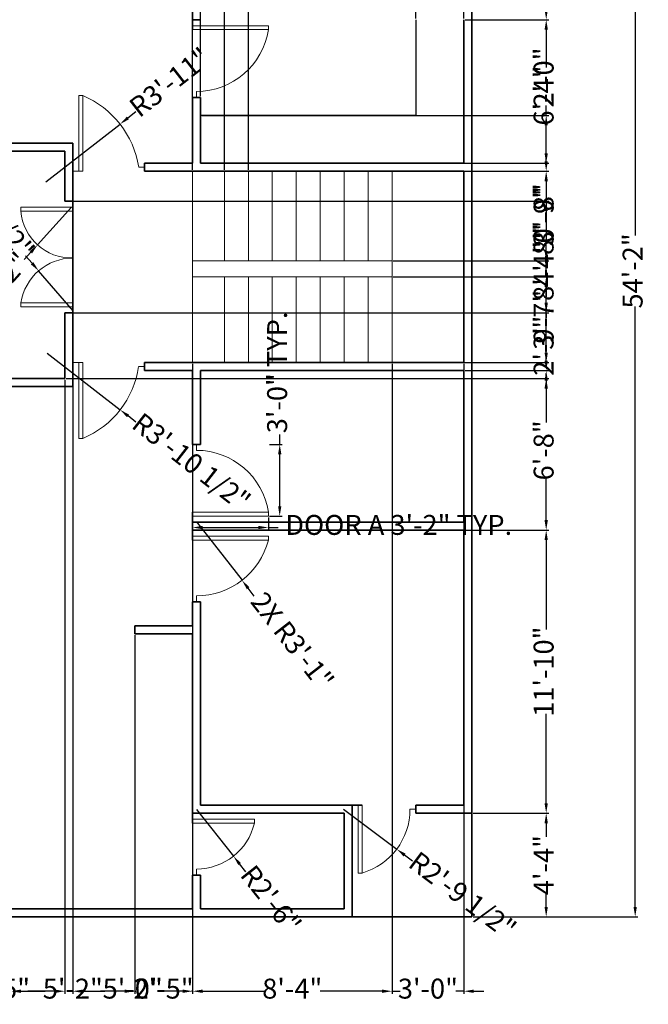
# Model space of a CAD drawing. Units: inches. Extents: x 2565 to 3182, y 2168 to 2957.
# Tile 2 of 3: x 2867 to 3182, y 2168 to 2662. Entities that reach past the tile are written whole.
import ezdxf

# ---------------------------------------------------------------- set-up
doc = ezdxf.new("R2010")
doc.units = ezdxf.units.IN
for name, color, linetype, lineweight in [('A-ANNO-DIMS', 2, 'Continuous', 13), ('A-DOOR', 4, 'Continuous', 18), ('A-FLOR-FIXT', 9, 'Continuous', 25), ('A-FLOR-STRS', 7, 'Continuous', 18), ('A-WALL', 7, 'Continuous', 35)]:
    doc.layers.add(name, color=color, linetype=linetype, lineweight=lineweight)
doc.styles.get("Standard").update_dxf_attribs({"font": 'arial.ttf'})
doc.dimstyles.new('ISO-25', dxfattribs={"dimtxt": 10, "dimasz": 5, "dimexe": 1.25, "dimexo": 0.625, "dimtad": 0, "dimdec": 0, "dimrnd": 10, "dimlunit": 3, "dimtxsty": 'Standard', "dimcen": 2.5, "dimadec": 0, "dimazin": 0, "dimtfac": 1, "dimtdec": 0, "dimtmove": 0, "dimatfit": 3, "dimfxl": 1, "dimarcsym": 0})

# ---------------------------------------------------------------- blocks, each defined once
blk = doc.blocks.new('*D2')
at = {"layer": 'A-ANNO-DIMS', "color": 0, "lineweight": -2, "transparency": 16777216}
for p, q in [((3094.05, 2859.77), (3176.57, 2859.77)), ((3175.32, 2854.77), (3175.32, 2553.57)), ((3175.32, 2216.77), (3175.32, 2517.97)), ((3094.05, 2211.77), (3176.57, 2211.77))]:
    blk.add_line(p, q, dxfattribs=at)
at = {"layer": 'A-ANNO-DIMS', "color": 0, "transparency": 16777216}
for points in [[(3174.49, 2854.77), (3176.15, 2854.77), (3175.32, 2859.77)], [(3174.49, 2216.77), (3176.15, 2216.77), (3175.32, 2211.77)]]:
    blk.add_solid(points, dxfattribs=at)
at = {"layer": 'Defpoints', "color": 0, "transparency": 16777216}
for p in [(3093.43, 2859.77), (3093.43, 2211.77), (3175.32, 2211.77)]:
    blk.add_point(p, dxfattribs=at)
at = {"layer": 'A-ANNO-DIMS', "color": 0, "transparency": 16777216, "insert": (3175.32, 2535.77), "char_height": 10, "attachment_point": 5, "rotation": 90}
blk.add_mtext('54\'-2"', dxfattribs=at)
blk = doc.blocks.new('DOOR-SWING-36-OPENING-39')
for p, q in [((2, 36), (2, 33)), ((38, 2), (0, 2)), ((0, 2), (0, 0)), ((2, 0), (38, 0)), ((38, 0), (38, 2))]:
    blk.add_line(p, q)
blk.add_arc((2, -3.4), 36.4, 8.5358, 90)
blk = doc.blocks.new('DOOR-SWING-36-OPENING-36')
for p, q in [((0, 2), (0, 38)), ((0, 38), (2, 38)), ((2, 38), (2, 0)), ((0, 0), (0, 2)), ((33, 2), (30, 2)), ((2, 0), (0, 0))]:
    blk.add_line(p, q)
blk.add_arc((-7.14, 2), 37.14, 0, 75.75)
blk = doc.blocks.new('*D7')
at = {"layer": 'A-ANNO-DIMS', "color": 0, "lineweight": -2, "transparency": 16777216}
for p, q in [((2953.43, 2412.14), (2953.43, 2405.82)), ((2991.43, 2412.14), (2991.43, 2405.82)), ((2958.43, 2407.07), (2986.43, 2407.07)), ((2991.43, 2407.07), (2996.43, 2407.07))]:
    blk.add_line(p, q, dxfattribs=at)
at = {"layer": 'A-ANNO-DIMS', "color": 0, "transparency": 16777216}
for points in [[(2958.43, 2407.9), (2958.43, 2406.23), (2953.43, 2407.07)], [(2986.43, 2407.9), (2986.43, 2406.23), (2991.43, 2407.07)]]:
    blk.add_solid(points, dxfattribs=at)
at = {"layer": 'Defpoints', "color": 0, "transparency": 16777216}
for p in [(2953.43, 2412.77), (2991.43, 2412.77), (2991.43, 2407.07)]:
    blk.add_point(p, dxfattribs=at)
at = {"layer": 'A-ANNO-DIMS', "color": 0, "transparency": 16777216, "insert": (3056.78, 2407.07), "char_height": 10, "attachment_point": 5}
blk.add_mtext('DOOR A 3\'-2" TYP.', dxfattribs=at)
blk = doc.blocks.new('*D8')
at = {"layer": 'A-ANNO-DIMS', "color": 0, "lineweight": -2, "transparency": 16777216}
for p, q in [((2997.13, 2448.77), (2997.13, 2453.77)), ((2992.05, 2448.77), (2998.38, 2448.77)), ((2997.13, 2417.77), (2997.13, 2443.77)), ((2992.05, 2412.77), (2998.38, 2412.77))]:
    blk.add_line(p, q, dxfattribs=at)
at = {"layer": 'A-ANNO-DIMS', "color": 0, "transparency": 16777216}
for points in [[(2996.3, 2443.77), (2997.96, 2443.77), (2997.13, 2448.77)], [(2996.3, 2417.77), (2997.96, 2417.77), (2997.13, 2412.77)]]:
    blk.add_solid(points, dxfattribs=at)
at = {"layer": 'Defpoints', "color": 0, "transparency": 16777216}
for p in [(2991.43, 2448.77), (2997.13, 2448.77), (2991.43, 2412.77)]:
    blk.add_point(p, dxfattribs=at)
at = {"layer": 'A-ANNO-DIMS', "color": 0, "transparency": 16777216, "insert": (2997.13, 2484.87), "char_height": 10, "attachment_point": 5, "rotation": 90}
blk.add_mtext('3\'-0" TYP.', dxfattribs=at)
blk = doc.blocks.new('*D29')
at = {"layer": 'A-ANNO-DIMS', "color": 0, "lineweight": -2, "transparency": 16777216}
for p, q in [((3094.05, 2263.77), (3131.96, 2263.77)), ((3130.71, 2258.77), (3130.71, 2251.89)), ((3130.71, 2216.77), (3130.71, 2223.65)), ((3094.05, 2211.77), (3131.96, 2211.77))]:
    blk.add_line(p, q, dxfattribs=at)
at = {"layer": 'A-ANNO-DIMS', "color": 0, "transparency": 16777216}
for points in [[(3129.88, 2258.77), (3131.54, 2258.77), (3130.71, 2263.77)], [(3129.88, 2216.77), (3131.54, 2216.77), (3130.71, 2211.77)]]:
    blk.add_solid(points, dxfattribs=at)
at = {"layer": 'Defpoints', "color": 0, "transparency": 16777216}
for p in [(3093.43, 2263.77), (3130.71, 2263.77), (3093.43, 2211.77)]:
    blk.add_point(p, dxfattribs=at)
at = {"layer": 'A-ANNO-DIMS', "color": 0, "transparency": 16777216, "insert": (3130.71, 2237.77), "char_height": 10, "attachment_point": 5, "rotation": 90}
blk.add_mtext('4\'-4"', dxfattribs=at)
blk = doc.blocks.new('*D30')
at = {"layer": 'A-ANNO-DIMS', "color": 0, "lineweight": -2, "transparency": 16777216}
for p, q in [((3090.05, 2405.77), (3131.96, 2405.77)), ((3130.71, 2400.77), (3130.71, 2355.98)), ((3130.71, 2268.77), (3130.71, 2313.55)), ((3094.05, 2263.77), (3131.96, 2263.77))]:
    blk.add_line(p, q, dxfattribs=at)
at = {"layer": 'A-ANNO-DIMS', "color": 0, "transparency": 16777216}
for points in [[(3129.88, 2400.77), (3131.54, 2400.77), (3130.71, 2405.77)], [(3129.88, 2268.77), (3131.54, 2268.77), (3130.71, 2263.77)]]:
    blk.add_solid(points, dxfattribs=at)
at = {"layer": 'Defpoints', "color": 0, "transparency": 16777216}
for p in [(3089.43, 2405.77), (3130.71, 2405.77), (3093.43, 2263.77)]:
    blk.add_point(p, dxfattribs=at)
at = {"layer": 'A-ANNO-DIMS', "color": 0, "transparency": 16777216, "insert": (3130.71, 2334.77), "char_height": 10, "attachment_point": 5, "rotation": 90}
blk.add_mtext('11\'-10"', dxfattribs=at)
blk = doc.blocks.new('*D31')
at = {"layer": 'A-ANNO-DIMS', "color": 0, "lineweight": -2, "transparency": 16777216}
for p, q in [((3090.05, 2485.77), (3131.96, 2485.77)), ((3130.71, 2480.77), (3130.71, 2459.71)), ((3130.71, 2410.77), (3130.71, 2431.82)), ((3090.05, 2405.77), (3131.96, 2405.77))]:
    blk.add_line(p, q, dxfattribs=at)
at = {"layer": 'A-ANNO-DIMS', "color": 0, "transparency": 16777216}
for points in [[(3129.88, 2480.77), (3131.54, 2480.77), (3130.71, 2485.77)], [(3129.88, 2410.77), (3131.54, 2410.77), (3130.71, 2405.77)]]:
    blk.add_solid(points, dxfattribs=at)
at = {"layer": 'Defpoints', "color": 0, "transparency": 16777216}
for p in [(3089.43, 2485.77), (3130.71, 2485.77), (3089.43, 2405.77)]:
    blk.add_point(p, dxfattribs=at)
at = {"layer": 'A-ANNO-DIMS', "color": 0, "transparency": 16777216, "insert": (3130.71, 2445.77), "char_height": 10, "attachment_point": 5, "rotation": 90}
blk.add_mtext('6\'-8"', dxfattribs=at)
blk = doc.blocks.new('*D32')
at = {"layer": 'A-ANNO-DIMS', "color": 0, "lineweight": -2, "transparency": 16777216}
for p, q in [((3090.05, 2585.77), (3131.96, 2585.77)), ((3130.71, 2580.77), (3130.71, 2549.69)), ((3130.71, 2490.77), (3130.71, 2521.84)), ((3090.05, 2485.77), (3131.96, 2485.77))]:
    blk.add_line(p, q, dxfattribs=at)
at = {"layer": 'A-ANNO-DIMS', "color": 0, "transparency": 16777216}
for points in [[(3129.88, 2580.77), (3131.54, 2580.77), (3130.71, 2585.77)], [(3129.88, 2490.77), (3131.54, 2490.77), (3130.71, 2485.77)]]:
    blk.add_solid(points, dxfattribs=at)
at = {"layer": 'Defpoints', "color": 0, "transparency": 16777216}
for p in [(3089.43, 2585.77), (3130.71, 2585.77), (3089.43, 2485.77)]:
    blk.add_point(p, dxfattribs=at)
at = {"layer": 'A-ANNO-DIMS', "color": 0, "transparency": 16777216, "insert": (3130.71, 2535.77), "char_height": 10, "attachment_point": 5, "rotation": 90}
blk.add_mtext('8\'-4"', dxfattribs=at)
blk = doc.blocks.new('*D33')
at = {"layer": 'A-ANNO-DIMS', "color": 0, "lineweight": -2, "transparency": 16777216}
for p, q in [((3090.05, 2661.77), (3131.96, 2661.77)), ((3130.71, 2656.77), (3130.71, 2637.71)), ((3130.71, 2590.77), (3130.71, 2609.82)), ((3090.05, 2585.77), (3131.96, 2585.77))]:
    blk.add_line(p, q, dxfattribs=at)
at = {"layer": 'A-ANNO-DIMS', "color": 0, "transparency": 16777216}
for points in [[(3129.88, 2656.77), (3131.54, 2656.77), (3130.71, 2661.77)], [(3129.88, 2590.77), (3131.54, 2590.77), (3130.71, 2585.77)]]:
    blk.add_solid(points, dxfattribs=at)
at = {"layer": 'Defpoints', "color": 0, "transparency": 16777216}
for p in [(3089.43, 2661.77), (3130.71, 2661.77), (3089.43, 2585.77)]:
    blk.add_point(p, dxfattribs=at)
at = {"layer": 'A-ANNO-DIMS', "color": 0, "transparency": 16777216, "insert": (3130.71, 2623.77), "char_height": 10, "attachment_point": 5, "rotation": 90}
blk.add_mtext('6\'-4"', dxfattribs=at)
blk = doc.blocks.new('*D34')
at = {"layer": 'A-ANNO-DIMS', "color": 0, "lineweight": -2, "transparency": 16777216}
for p, q in [((3090.05, 2803.77), (3131.96, 2803.77)), ((3130.71, 2798.77), (3130.71, 2753.98)), ((3130.71, 2666.77), (3130.71, 2711.55)), ((3090.05, 2661.77), (3131.96, 2661.77))]:
    blk.add_line(p, q, dxfattribs=at)
at = {"layer": 'A-ANNO-DIMS', "color": 0, "transparency": 16777216}
for points in [[(3129.88, 2798.77), (3131.54, 2798.77), (3130.71, 2803.77)], [(3129.88, 2666.77), (3131.54, 2666.77), (3130.71, 2661.77)]]:
    blk.add_solid(points, dxfattribs=at)
at = {"layer": 'Defpoints', "color": 0, "transparency": 16777216}
for p in [(3089.43, 2803.77), (3130.71, 2803.77), (3089.43, 2661.77)]:
    blk.add_point(p, dxfattribs=at)
at = {"layer": 'A-ANNO-DIMS', "color": 0, "transparency": 16777216, "insert": (3130.71, 2732.77), "char_height": 10, "attachment_point": 5, "rotation": 90}
blk.add_mtext('11\'-10"', dxfattribs=at)
blk = doc.blocks.new('*D37')
at = {"layer": 'A-ANNO-DIMS', "color": 0, "lineweight": -2, "transparency": 16777216}
for p, q in [((2924.43, 2353.14), (2924.43, 2173.24)), ((2953.43, 2353.14), (2953.43, 2173.24)), ((2919.43, 2174.49), (2914.43, 2174.49)), ((2924.43, 2174.49), (2924.93, 2174.49)), ((2953.43, 2174.49), (2952.93, 2174.49)), ((2958.43, 2174.49), (2963.43, 2174.49))]:
    blk.add_line(p, q, dxfattribs=at)
at = {"layer": 'A-ANNO-DIMS', "color": 0, "transparency": 16777216}
for points in [[(2919.43, 2175.32), (2919.43, 2173.65), (2924.43, 2174.49)], [(2958.43, 2175.32), (2958.43, 2173.65), (2953.43, 2174.49)]]:
    blk.add_solid(points, dxfattribs=at)
at = {"layer": 'Defpoints', "color": 0, "transparency": 16777216}
for p in [(2924.43, 2353.77), (2953.43, 2353.77), (2953.43, 2174.49)]:
    blk.add_point(p, dxfattribs=at)
at = {"layer": 'A-ANNO-DIMS', "color": 0, "transparency": 16777216, "insert": (2938.93, 2174.49), "char_height": 10, "attachment_point": 5}
blk.add_mtext('2\'-5"', dxfattribs=at)
blk = doc.blocks.new('*D38')
at = {"layer": 'A-ANNO-DIMS', "color": 0, "lineweight": -2, "transparency": 16777216}
for p, q in [((2862.43, 2353.14), (2862.43, 2173.24)), ((2924.43, 2353.14), (2924.43, 2173.24)), ((2867.43, 2174.49), (2879.51, 2174.49)), ((2919.43, 2174.49), (2907.35, 2174.49))]:
    blk.add_line(p, q, dxfattribs=at)
at = {"layer": 'A-ANNO-DIMS', "color": 0, "transparency": 16777216}
for points in [[(2867.43, 2175.32), (2867.43, 2173.65), (2862.43, 2174.49)], [(2919.43, 2175.32), (2919.43, 2173.65), (2924.43, 2174.49)]]:
    blk.add_solid(points, dxfattribs=at)
at = {"layer": 'Defpoints', "color": 0, "transparency": 16777216}
for p in [(2862.43, 2353.77), (2924.43, 2353.77), (2924.43, 2174.49)]:
    blk.add_point(p, dxfattribs=at)
at = {"layer": 'A-ANNO-DIMS', "color": 0, "transparency": 16777216, "insert": (2893.43, 2174.49), "char_height": 10, "attachment_point": 5}
blk.add_mtext('5\'-2"', dxfattribs=at)
blk = doc.blocks.new('*D45')
at = {"layer": 'A-ANNO-DIMS', "color": 0, "lineweight": -2, "transparency": 16777216}
for p, q in [((3130.71, 2519.77), (3130.71, 2524.77)), ((2890.05, 2514.77), (3131.96, 2514.77)), ((3130.71, 2514.77), (3130.71, 2512.27)), ((3130.71, 2481.77), (3130.71, 2484.27)), ((2890.05, 2481.77), (3131.96, 2481.77)), ((3130.71, 2476.77), (3130.71, 2471.77))]:
    blk.add_line(p, q, dxfattribs=at)
at = {"layer": 'A-ANNO-DIMS', "color": 0, "transparency": 16777216}
for points in [[(3129.88, 2519.77), (3131.54, 2519.77), (3130.71, 2514.77)], [(3129.88, 2476.77), (3131.54, 2476.77), (3130.71, 2481.77)]]:
    blk.add_solid(points, dxfattribs=at)
at = {"layer": 'Defpoints', "color": 0, "transparency": 16777216}
for p in [(2889.43, 2514.77), (3130.71, 2514.77), (2889.43, 2481.77)]:
    blk.add_point(p, dxfattribs=at)
at = {"layer": 'A-ANNO-DIMS', "color": 0, "transparency": 16777216, "insert": (3130.71, 2498.27), "char_height": 10, "attachment_point": 5, "rotation": 90}
blk.add_mtext('2\'-9"', dxfattribs=at)
blk = doc.blocks.new('*D46')
at = {"layer": 'A-ANNO-DIMS', "color": 0, "lineweight": -2, "transparency": 16777216}
for p, q in [((2890.05, 2570.77), (3131.96, 2570.77)), ((3130.71, 2565.77), (3130.71, 2556.89)), ((3130.71, 2519.77), (3130.71, 2528.65)), ((2890.05, 2514.77), (3131.96, 2514.77))]:
    blk.add_line(p, q, dxfattribs=at)
at = {"layer": 'A-ANNO-DIMS', "color": 0, "transparency": 16777216}
for points in [[(3129.88, 2565.77), (3131.54, 2565.77), (3130.71, 2570.77)], [(3129.88, 2519.77), (3131.54, 2519.77), (3130.71, 2514.77)]]:
    blk.add_solid(points, dxfattribs=at)
at = {"layer": 'Defpoints', "color": 0, "transparency": 16777216}
for p in [(2889.43, 2570.77), (3130.71, 2570.77), (2889.43, 2514.77)]:
    blk.add_point(p, dxfattribs=at)
at = {"layer": 'A-ANNO-DIMS', "color": 0, "transparency": 16777216, "insert": (3130.71, 2542.77), "char_height": 10, "attachment_point": 5, "rotation": 90}
blk.add_mtext('4\'-8"', dxfattribs=at)
blk = doc.blocks.new('*D48')
at = {"layer": 'A-ANNO-DIMS', "color": 0, "lineweight": -2, "transparency": 16777216}
for p, q in [((2824.43, 2481.14), (2824.43, 2173.24)), ((2889.43, 2481.14), (2889.43, 2173.24)), ((2829.43, 2174.49), (2843.01, 2174.49)), ((2884.43, 2174.49), (2870.85, 2174.49))]:
    blk.add_line(p, q, dxfattribs=at)
at = {"layer": 'A-ANNO-DIMS', "color": 0, "transparency": 16777216}
for points in [[(2829.43, 2175.32), (2829.43, 2173.65), (2824.43, 2174.49)], [(2884.43, 2175.32), (2884.43, 2173.65), (2889.43, 2174.49)]]:
    blk.add_solid(points, dxfattribs=at)
at = {"layer": 'Defpoints', "color": 0, "transparency": 16777216}
for p in [(2824.43, 2481.77), (2889.43, 2481.77), (2889.43, 2174.49)]:
    blk.add_point(p, dxfattribs=at)
at = {"layer": 'A-ANNO-DIMS', "color": 0, "transparency": 16777216, "insert": (2856.93, 2174.49), "char_height": 10, "attachment_point": 5}
blk.add_mtext('5\'-5"', dxfattribs=at)
blk = doc.blocks.new('*D49')
at = {"layer": 'A-ANNO-DIMS', "color": 0, "lineweight": -2, "transparency": 16777216}
for p, q in [((2893.43, 2489.14), (2893.43, 2173.24)), ((2953.43, 2489.14), (2953.43, 2173.24)), ((2898.43, 2174.49), (2909.51, 2174.49)), ((2948.43, 2174.49), (2937.35, 2174.49))]:
    blk.add_line(p, q, dxfattribs=at)
at = {"layer": 'A-ANNO-DIMS', "color": 0, "transparency": 16777216}
for points in [[(2898.43, 2175.32), (2898.43, 2173.65), (2893.43, 2174.49)], [(2948.43, 2175.32), (2948.43, 2173.65), (2953.43, 2174.49)]]:
    blk.add_solid(points, dxfattribs=at)
at = {"layer": 'Defpoints', "color": 0, "transparency": 16777216}
for p in [(2893.43, 2489.77), (2953.43, 2489.77), (2953.43, 2174.49)]:
    blk.add_point(p, dxfattribs=at)
at = {"layer": 'A-ANNO-DIMS', "color": 0, "transparency": 16777216, "insert": (2923.43, 2174.49), "char_height": 10, "attachment_point": 5}
blk.add_mtext('5\'-0"', dxfattribs=at)
blk = doc.blocks.new('*D50')
at = {"layer": 'A-ANNO-DIMS', "color": 0, "lineweight": -2, "transparency": 16777216}
for p, q in [((2953.43, 2489.14), (2953.43, 2173.24)), ((3053.43, 2489.14), (3053.43, 2173.24)), ((2958.43, 2174.49), (2989.51, 2174.49)), ((3048.43, 2174.49), (3017.35, 2174.49))]:
    blk.add_line(p, q, dxfattribs=at)
at = {"layer": 'A-ANNO-DIMS', "color": 0, "transparency": 16777216}
for points in [[(2958.43, 2175.32), (2958.43, 2173.65), (2953.43, 2174.49)], [(3048.43, 2175.32), (3048.43, 2173.65), (3053.43, 2174.49)]]:
    blk.add_solid(points, dxfattribs=at)
at = {"layer": 'Defpoints', "color": 0, "transparency": 16777216}
for p in [(2953.43, 2489.77), (3053.43, 2489.77), (3053.43, 2174.49)]:
    blk.add_point(p, dxfattribs=at)
at = {"layer": 'A-ANNO-DIMS', "color": 0, "transparency": 16777216, "insert": (3003.43, 2174.49), "char_height": 10, "attachment_point": 5}
blk.add_mtext('8\'-4"', dxfattribs=at)
blk = doc.blocks.new('*D51')
at = {"layer": 'A-ANNO-DIMS', "color": 0, "lineweight": -2, "transparency": 16777216}
for p, q in [((3053.43, 2489.14), (3053.43, 2173.24)), ((3089.43, 2489.14), (3089.43, 2173.24)), ((3048.43, 2174.49), (3043.43, 2174.49)), ((3053.43, 2174.49), (3057.52, 2174.49)), ((3089.43, 2174.49), (3085.34, 2174.49)), ((3094.43, 2174.49), (3099.43, 2174.49))]:
    blk.add_line(p, q, dxfattribs=at)
at = {"layer": 'A-ANNO-DIMS', "color": 0, "transparency": 16777216}
for points in [[(3048.43, 2175.32), (3048.43, 2173.65), (3053.43, 2174.49)], [(3094.43, 2175.32), (3094.43, 2173.65), (3089.43, 2174.49)]]:
    blk.add_solid(points, dxfattribs=at)
at = {"layer": 'Defpoints', "color": 0, "transparency": 16777216}
for p in [(3053.43, 2489.77), (3089.43, 2489.77), (3089.43, 2174.49)]:
    blk.add_point(p, dxfattribs=at)
at = {"layer": 'A-ANNO-DIMS', "color": 0, "transparency": 16777216, "insert": (3071.43, 2174.49), "char_height": 10, "attachment_point": 5}
blk.add_mtext('3\'-0"', dxfattribs=at)
blk = doc.blocks.new('*D52')
at = {"layer": 'A-ANNO-DIMS', "color": 0, "lineweight": -2, "transparency": 16777216}
for p, q in [((2953.43, 2586.39), (2953.43, 2898.3)), ((2958.43, 2897.05), (2964.43, 2897.05)), ((2969.43, 2586.39), (2969.43, 2898.3)), ((2969.43, 2897.05), (2974.43, 2897.05))]:
    blk.add_line(p, q, dxfattribs=at)
at = {"layer": 'A-ANNO-DIMS', "color": 0, "transparency": 16777216}
for points in [[(2958.43, 2897.88), (2958.43, 2896.21), (2953.43, 2897.05)], [(2964.43, 2897.88), (2964.43, 2896.21), (2969.43, 2897.05)]]:
    blk.add_solid(points, dxfattribs=at)
at = {"layer": 'Defpoints', "color": 0, "transparency": 16777216}
for p in [(2969.43, 2897.05), (2953.43, 2585.77), (2969.43, 2585.77)]:
    blk.add_point(p, dxfattribs=at)
at = {"layer": 'A-ANNO-DIMS', "color": 0, "transparency": 16777216, "insert": (2987.87, 2897.05), "char_height": 10, "attachment_point": 5}
blk.add_mtext('1\'-4"', dxfattribs=at)
blk = doc.blocks.new('*D53')
at = {"layer": 'A-ANNO-DIMS', "color": 0, "lineweight": -2, "transparency": 16777216}
for p, q in [((2969.43, 2586.39), (2969.43, 2898.3)), ((2974.43, 2897.05), (2976.43, 2897.05)), ((2981.43, 2586.39), (2981.43, 2898.3)), ((2981.43, 2897.05), (2986.43, 2897.05))]:
    blk.add_line(p, q, dxfattribs=at)
at = {"layer": 'A-ANNO-DIMS', "color": 0, "transparency": 16777216}
for points in [[(2974.43, 2897.88), (2974.43, 2896.21), (2969.43, 2897.05)], [(2976.43, 2897.88), (2976.43, 2896.21), (2981.43, 2897.05)]]:
    blk.add_solid(points, dxfattribs=at)
at = {"layer": 'Defpoints', "color": 0, "transparency": 16777216}
for p in [(2981.43, 2897.05), (2969.43, 2585.77), (2981.43, 2585.77)]:
    blk.add_point(p, dxfattribs=at)
at = {"layer": 'A-ANNO-DIMS', "color": 0, "transparency": 16777216, "insert": (2999.87, 2897.05), "char_height": 10, "attachment_point": 5}
blk.add_mtext('1\'-0"', dxfattribs=at)
blk = doc.blocks.new('*D54')
at = {"layer": 'A-ANNO-DIMS', "color": 0, "lineweight": -2, "transparency": 16777216}
for p, q in [((3054.05, 2532.77), (3131.96, 2532.77)), ((3130.71, 2527.77), (3130.71, 2525.18)), ((3130.71, 2494.77), (3130.71, 2497.36)), ((3054.05, 2489.77), (3131.96, 2489.77))]:
    blk.add_line(p, q, dxfattribs=at)
at = {"layer": 'A-ANNO-DIMS', "color": 0, "transparency": 16777216}
for points in [[(3129.88, 2527.77), (3131.54, 2527.77), (3130.71, 2532.77)], [(3129.88, 2494.77), (3131.54, 2494.77), (3130.71, 2489.77)]]:
    blk.add_solid(points, dxfattribs=at)
at = {"layer": 'Defpoints', "color": 0, "transparency": 16777216}
for p in [(3053.43, 2532.77), (3130.71, 2532.77), (3053.43, 2489.77)]:
    blk.add_point(p, dxfattribs=at)
at = {"layer": 'A-ANNO-DIMS', "color": 0, "transparency": 16777216, "insert": (3130.71, 2511.27), "char_height": 10, "attachment_point": 5, "rotation": 90}
blk.add_mtext('3\'-7"', dxfattribs=at)
blk = doc.blocks.new('*D55')
at = {"layer": 'A-ANNO-DIMS', "color": 0, "lineweight": -2, "transparency": 16777216}
for p, q in [((3130.71, 2545.77), (3130.71, 2550.77)), ((3054.05, 2540.77), (3131.96, 2540.77)), ((3130.71, 2532.77), (3130.71, 2540.77)), ((3054.05, 2532.77), (3131.96, 2532.77)), ((3130.71, 2527.77), (3130.71, 2522.77))]:
    blk.add_line(p, q, dxfattribs=at)
at = {"layer": 'A-ANNO-DIMS', "color": 0, "transparency": 16777216}
for points in [[(3129.88, 2545.77), (3131.54, 2545.77), (3130.71, 2540.77)], [(3129.88, 2527.77), (3131.54, 2527.77), (3130.71, 2532.77)]]:
    blk.add_solid(points, dxfattribs=at)
at = {"layer": 'Defpoints', "color": 0, "transparency": 16777216}
for p in [(3053.43, 2540.77), (3130.71, 2540.77), (3053.43, 2532.77)]:
    blk.add_point(p, dxfattribs=at)
at = {"layer": 'A-ANNO-DIMS', "color": 0, "transparency": 16777216, "insert": (3130.71, 2564.68), "char_height": 10, "attachment_point": 5, "rotation": 90}
blk.add_mtext('0\'-8"', dxfattribs=at)
blk = doc.blocks.new('*D56')
at = {"layer": 'A-ANNO-DIMS', "color": 0, "lineweight": -2, "transparency": 16777216}
for p, q in [((3054.05, 2585.77), (3131.96, 2585.77)), ((3130.71, 2580.77), (3130.71, 2577.18)), ((3130.71, 2545.77), (3130.71, 2549.36)), ((3054.05, 2540.77), (3131.96, 2540.77))]:
    blk.add_line(p, q, dxfattribs=at)
at = {"layer": 'A-ANNO-DIMS', "color": 0, "transparency": 16777216}
for points in [[(3129.88, 2580.77), (3131.54, 2580.77), (3130.71, 2585.77)], [(3129.88, 2545.77), (3131.54, 2545.77), (3130.71, 2540.77)]]:
    blk.add_solid(points, dxfattribs=at)
at = {"layer": 'Defpoints', "color": 0, "transparency": 16777216}
for p in [(3053.43, 2585.77), (3130.71, 2585.77), (3053.43, 2540.77)]:
    blk.add_point(p, dxfattribs=at)
at = {"layer": 'A-ANNO-DIMS', "color": 0, "transparency": 16777216, "insert": (3130.71, 2563.27), "char_height": 10, "attachment_point": 5, "rotation": 90}
blk.add_mtext('3\'-9"', dxfattribs=at)
blk = doc.blocks.new('*D57')
at = {"layer": 'A-ANNO-DIMS', "color": 0, "lineweight": -2, "transparency": 16777216}
for p, q in [((3065.43, 2662.39), (3065.43, 2898.3)), ((3070.43, 2897.05), (3084.43, 2897.05)), ((3089.43, 2662.39), (3089.43, 2898.3)), ((3089.43, 2897.05), (3094.43, 2897.05))]:
    blk.add_line(p, q, dxfattribs=at)
at = {"layer": 'A-ANNO-DIMS', "color": 0, "transparency": 16777216}
for points in [[(3070.43, 2897.88), (3070.43, 2896.21), (3065.43, 2897.05)], [(3084.43, 2897.88), (3084.43, 2896.21), (3089.43, 2897.05)]]:
    blk.add_solid(points, dxfattribs=at)
at = {"layer": 'Defpoints', "color": 0, "transparency": 16777216}
for p in [(3089.43, 2897.05), (3065.43, 2661.77), (3089.43, 2661.77)]:
    blk.add_point(p, dxfattribs=at)
at = {"layer": 'A-ANNO-DIMS', "color": 0, "transparency": 16777216, "insert": (3108.43, 2897.05), "char_height": 10, "attachment_point": 5}
blk.add_mtext('2\'-0"', dxfattribs=at)
blk = doc.blocks.new('*D58')
at = {"layer": 'A-ANNO-DIMS', "color": 0, "lineweight": -2, "transparency": 16777216}
for p, q in [((3130.71, 2613.77), (3130.71, 2618.77)), ((2958.05, 2613.77), (3131.96, 2613.77)), ((3130.71, 2594.77), (3130.71, 2608.77)), ((2958.05, 2589.77), (3131.96, 2589.77))]:
    blk.add_line(p, q, dxfattribs=at)
at = {"layer": 'A-ANNO-DIMS', "color": 0, "transparency": 16777216}
for points in [[(3129.88, 2608.77), (3131.54, 2608.77), (3130.71, 2613.77)], [(3129.88, 2594.77), (3131.54, 2594.77), (3130.71, 2589.77)]]:
    blk.add_solid(points, dxfattribs=at)
at = {"layer": 'Defpoints', "color": 0, "transparency": 16777216}
for p in [(2957.43, 2613.77), (3130.71, 2613.77), (2957.43, 2589.77)]:
    blk.add_point(p, dxfattribs=at)
at = {"layer": 'A-ANNO-DIMS', "color": 0, "transparency": 16777216, "insert": (3130.71, 2632.77), "char_height": 10, "attachment_point": 5, "rotation": 90}
blk.add_mtext('2\'-0"', dxfattribs=at)
blk = doc.blocks.new('*D59')
at = {"layer": 'A-ANNO-DIMS', "color": 0, "lineweight": -2, "transparency": 16777216}
for p, q in [((2948.43, 2897.05), (2943.43, 2897.05)), ((2953.43, 2623.39), (2953.43, 2898.3)), ((2953.43, 2897.05), (2957.43, 2897.05)), ((2957.43, 2623.39), (2957.43, 2898.3)), ((2962.43, 2897.05), (2967.43, 2897.05))]:
    blk.add_line(p, q, dxfattribs=at)
at = {"layer": 'A-ANNO-DIMS', "color": 0, "transparency": 16777216}
for points in [[(2948.43, 2897.88), (2948.43, 2896.21), (2953.43, 2897.05)], [(2962.43, 2897.88), (2962.43, 2896.21), (2957.43, 2897.05)]]:
    blk.add_solid(points, dxfattribs=at)
at = {"layer": 'Defpoints', "color": 0, "transparency": 16777216}
for p in [(2957.43, 2897.05), (2953.43, 2622.77), (2957.43, 2622.77)]:
    blk.add_point(p, dxfattribs=at)
at = {"layer": 'A-ANNO-DIMS', "color": 0, "transparency": 16777216, "insert": (2981.35, 2897.05), "char_height": 10, "attachment_point": 5}
blk.add_mtext('0\'-4"', dxfattribs=at)
blk = doc.blocks.new('*D60')
at = {"layer": 'A-ANNO-DIMS', "color": 0, "lineweight": -2, "transparency": 16777216}
for p, q in [((2924.97, 2615.52), (2921.02, 2612.45)), ((2879.89, 2580.46), (2917.08, 2609.38))]:
    blk.add_line(p, q, dxfattribs=at)
at = {"layer": 'A-ANNO-DIMS', "color": 0, "transparency": 16777216}
blk.add_solid([(2920.51, 2613.11), (2921.53, 2611.79), (2917.08, 2609.38)], dxfattribs=at)
at = {"layer": 'Defpoints', "color": 0, "transparency": 16777216}
for p in [(2917.08, 2609.38), (2879.89, 2580.46)]:
    blk.add_point(p, dxfattribs=at)
at = {"layer": 'A-ANNO-DIMS', "color": 0, "transparency": 16777216, "insert": (2942.8, 2629.39), "char_height": 10, "attachment_point": 5, "rotation": 37.8749}
blk.add_mtext('R3\'-11"', dxfattribs=at)
blk = doc.blocks.new('*D61')
at = {"layer": 'A-ANNO-DIMS', "color": 0, "lineweight": -2, "transparency": 16777216}
for p, q in [((2880.6, 2494.52), (2917.17, 2466.08)), ((2925.06, 2459.94), (2921.11, 2463.01))]:
    blk.add_line(p, q, dxfattribs=at)
at = {"layer": 'A-ANNO-DIMS', "color": 0, "transparency": 16777216}
blk.add_solid([(2921.63, 2463.67), (2920.6, 2462.36), (2917.17, 2466.08)], dxfattribs=at)
at = {"layer": 'Defpoints', "color": 0, "transparency": 16777216}
for p in [(2880.6, 2494.52), (2917.17, 2466.08)]:
    blk.add_point(p, dxfattribs=at)
at = {"layer": 'A-ANNO-DIMS', "color": 0, "transparency": 16777216, "insert": (2952.09, 2438.92), "char_height": 10, "attachment_point": 5, "rotation": 322.1251}
blk.add_mtext('R3\'-10 1/2"', dxfattribs=at)
blk = doc.blocks.new('*D62')
at = {"layer": 'A-ANNO-DIMS', "color": 0, "lineweight": -2, "transparency": 16777216}
for p, q in [((2955.43, 2409.91), (2978.23, 2380.59)), ((2984.37, 2372.7), (2981.3, 2376.65))]:
    blk.add_line(p, q, dxfattribs=at)
at = {"layer": 'A-ANNO-DIMS', "color": 0, "transparency": 16777216}
blk.add_solid([(2981.96, 2377.16), (2980.64, 2376.13), (2978.23, 2380.59)], dxfattribs=at)
at = {"layer": 'Defpoints', "color": 0, "transparency": 16777216}
for p in [(2955.43, 2409.91), (2978.23, 2380.59)]:
    blk.add_point(p, dxfattribs=at)
at = {"layer": 'A-ANNO-DIMS', "color": 0, "transparency": 16777216, "insert": (3002.5, 2349.39), "char_height": 10, "attachment_point": 5, "rotation": 307.8754}
blk.add_mtext('2X R3\'-1"', dxfattribs=at)
blk = doc.blocks.new('*D64')
at = {"layer": 'A-ANNO-DIMS', "color": 0, "lineweight": -2, "transparency": 16777216}
for p, q in [((3029.1, 2265.77), (3055.76, 2245.77)), ((3063.76, 2239.77), (3059.76, 2242.77))]:
    blk.add_line(p, q, dxfattribs=at)
at = {"layer": 'A-ANNO-DIMS', "color": 0, "transparency": 16777216}
blk.add_solid([(3060.26, 2243.43), (3059.26, 2242.1), (3055.76, 2245.77)], dxfattribs=at)
at = {"layer": 'Defpoints', "color": 0, "transparency": 16777216}
for p in [(3029.1, 2265.77), (3055.76, 2245.77)]:
    blk.add_point(p, dxfattribs=at)
at = {"layer": 'A-ANNO-DIMS', "color": 0, "transparency": 16777216, "insert": (3088.04, 2221.56), "char_height": 10, "attachment_point": 5, "rotation": 323.1298}
blk.add_mtext('R2\'-9 1/2"', dxfattribs=at)
blk = doc.blocks.new('*D66')
at = {"layer": 'A-ANNO-DIMS', "color": 0, "lineweight": -2, "transparency": 16777216}
for p, q in [((2955.43, 2265.55), (2973.94, 2242.22)), ((2980.15, 2234.38), (2977.04, 2238.3))]:
    blk.add_line(p, q, dxfattribs=at)
at = {"layer": 'A-ANNO-DIMS', "color": 0, "transparency": 16777216}
blk.add_solid([(2977.7, 2238.82), (2976.39, 2237.78), (2973.94, 2242.22)], dxfattribs=at)
at = {"layer": 'Defpoints', "color": 0, "transparency": 16777216}
for p in [(2955.43, 2265.55), (2973.94, 2242.22)]:
    blk.add_point(p, dxfattribs=at)
at = {"layer": 'A-ANNO-DIMS', "color": 0, "transparency": 16777216, "insert": (2991.77, 2219.73), "char_height": 10, "attachment_point": 5, "rotation": 308.4183}
blk.add_mtext('R2\'-6"', dxfattribs=at)
blk = doc.blocks.new('*D70')
at = {"layer": 'A-ANNO-DIMS', "color": 0, "lineweight": -2, "transparency": 16777216}
for p, q in [((2869.74, 2543.36), (2873.01, 2539.58)), ((2893.6, 2515.77), (2876.29, 2535.8))]:
    blk.add_line(p, q, dxfattribs=at)
at = {"layer": 'A-ANNO-DIMS', "color": 0, "transparency": 16777216}
blk.add_solid([(2873.65, 2540.13), (2872.38, 2539.04), (2876.29, 2535.8)], dxfattribs=at)
at = {"layer": 'Defpoints', "color": 0, "transparency": 16777216}
for p in [(2876.29, 2535.8), (2893.6, 2515.77)]:
    blk.add_point(p, dxfattribs=at)
at = {"layer": 'A-ANNO-DIMS', "color": 0, "transparency": 16777216, "insert": (2849.89, 2566.32), "char_height": 10, "attachment_point": 5, "rotation": 310.8471}
blk.add_mtext('R2\'-2 1/2"', dxfattribs=at)
blk = doc.blocks.new('*D72')
at = {"layer": 'A-ANNO-DIMS', "color": 0, "lineweight": -2, "transparency": 16777216}
for p, q in [((2892.82, 2567.71), (2875.74, 2548.82)), ((2869.03, 2541.41), (2872.38, 2545.11))]:
    blk.add_line(p, q, dxfattribs=at)
at = {"layer": 'A-ANNO-DIMS', "color": 0, "transparency": 16777216}
blk.add_solid([(2871.76, 2545.67), (2873, 2544.55), (2875.74, 2548.82)], dxfattribs=at)
at = {"layer": 'Defpoints', "color": 0, "transparency": 16777216}
for p in [(2892.82, 2567.71), (2875.74, 2548.82)]:
    blk.add_point(p, dxfattribs=at)
at = {"layer": 'A-ANNO-DIMS', "color": 0, "transparency": 16777216, "insert": (2848.67, 2518.9), "char_height": 10, "attachment_point": 5, "rotation": 47.8657}
blk.add_mtext('R2\'-1 1/2"', dxfattribs=at)

msp = doc.modelspace()

# ---------------------------------------------------------------- linework, layer by layer
at = {"layer": 'A-DOOR'}
for p, q in [((2953.43, 2658.77), (2956.22, 2658.77)), ((2896.43, 2587.77), (2896.43, 2623.77)), ((2896.43, 2623.77), (2898.43, 2623.77)), ((2898.43, 2623.77), (2898.43, 2587.77)), ((2896.43, 2587.77), (2896.43, 2585.77)), ((2898.43, 2587.77), (2898.43, 2585.77)), ((2929.43, 2587.77), (2926.43, 2587.77)), ((2898.43, 2585.77), (2893.43, 2585.77)), ((2893.43, 2585.77), (2896.43, 2585.77)), ((2891.43, 2567.77), (2867.43, 2567.77)), ((2867.43, 2567.77), (2867.43, 2565.77)), ((2867.43, 2565.77), (2893.43, 2565.77)), ((2891.43, 2567.77), (2893.43, 2567.77)), ((2891.43, 2542.25), (2891.43, 2542.25)), ((2867.43, 2517.77), (2867.43, 2519.77)), ((2867.43, 2519.77), (2893.43, 2519.77)), ((2891.43, 2517.77), (2867.43, 2517.77)), ((2891.43, 2517.77), (2893.43, 2517.77)), ((2898.43, 2489.77), (2893.43, 2489.77)), ((2893.43, 2489.77), (2896.43, 2489.77)), ((2896.43, 2489.77), (2896.43, 2487.45)), ((2898.43, 2451.77), (2898.43, 2489.77)), ((2896.43, 2487.77), (2896.43, 2451.77)), ((2929.43, 2487.77), (2926.43, 2487.77)), ((2896.43, 2451.77), (2898.43, 2451.77)), ((2953.43, 2412.77), (2957.43, 2412.77)), ((3038.43, 2267.77), (3036.43, 2267.77)), ((3036.43, 2267.77), (3036.43, 2265.77)), ((3038.43, 2233.77), (3038.43, 2267.77)), ((3036.43, 2265.77), (3036.43, 2233.77)), ((3065.43, 2265.77), (3062.43, 2265.77)), ((2953.43, 2258.77), (2953.43, 2260.77)), ((2953.43, 2260.77), (2958.84, 2260.77)), ((2984.43, 2258.77), (2953.43, 2258.77)), ((2955.43, 2260.77), (2984.43, 2260.77)), ((2984.43, 2260.77), (2984.43, 2258.77)), ((2955.43, 2232.77), (2955.43, 2235.77)), ((3036.43, 2233.77), (3038.43, 2233.77))]:
    msp.add_line(p, q, dxfattribs=at)
for centre, radius, start, end in [((2879.89, 2580.46), 47.11, 8.9244, 66.8256), ((2892.82, 2567.71), 25.47, 184.3654, 271.3666), ((2893.6, 2515.77), 26.47, 90.3709, 171.3214), ((2880.6, 2494.52), 46.32, 292.633, 351.617), ((3029.1, 2265.77), 33.33, 286.2602, 0), ((2955.43, 2265.55), 29.78, 270, 346.8361)]:
    msp.add_arc(centre, radius, start, end, dxfattribs=at)
at = {"layer": 'A-FLOR-FIXT'}
for p, q in [((3065.43, 2661.77), (3065.43, 2613.77)), ((3065.43, 2613.77), (2957.43, 2613.77))]:
    msp.add_line(p, q, dxfattribs=at)
at = {"layer": 'A-FLOR-STRS'}
for p, q in [((2953.43, 2585.77), (2953.43, 2489.77)), ((2953.43, 2585.77), (2953.43, 2489.77)), ((2969.43, 2585.77), (2969.43, 2540.77)), ((2981.43, 2585.77), (2981.43, 2540.77)), ((2993.43, 2585.77), (2993.43, 2540.77)), ((3005.43, 2585.77), (3005.43, 2540.77)), ((3017.43, 2585.77), (3017.43, 2540.77)), ((3029.43, 2585.77), (3029.43, 2540.77)), ((3041.43, 2585.77), (3041.43, 2540.77)), ((3053.43, 2585.77), (3053.43, 2540.77)), ((2957.43, 2540.77), (2953.43, 2540.77)), ((2953.43, 2540.77), (2953.43, 2532.77)), ((3053.43, 2540.77), (2957.43, 2540.77)), ((3053.43, 2532.77), (3053.43, 2540.77)), ((2953.43, 2532.77), (2957.43, 2532.77)), ((3053.43, 2532.77), (2957.43, 2532.77)), ((2969.43, 2532.77), (2969.43, 2489.77)), ((2981.43, 2532.77), (2981.43, 2489.77)), ((2993.43, 2532.77), (2993.43, 2489.77)), ((3005.43, 2532.77), (3005.43, 2489.77)), ((3017.43, 2532.77), (3017.43, 2489.77)), ((3029.43, 2532.77), (3029.43, 2489.77)), ((3041.43, 2532.77), (3041.43, 2489.77)), ((3053.43, 2532.77), (3053.43, 2489.77))]:
    msp.add_line(p, q, dxfattribs=at)
at = {"layer": 'A-WALL'}
for p, q in [((3093.43, 2211.77), (3093.43, 2859.77)), ((2953.43, 2670.77), (2953.43, 2656.77)), ((2957.43, 2661.77), (2953.43, 2661.77)), ((3089.43, 2589.77), (3089.43, 2661.77)), ((3089.43, 2661.77), (3089.43, 2589.77)), ((2957.43, 2622.77), (2953.43, 2622.77)), ((2953.43, 2622.77), (2953.43, 2589.77)), ((2957.43, 2622.77), (2957.43, 2589.77)), ((2893.43, 2599.77), (2833.43, 2599.77)), ((2893.43, 2599.77), (2889.43, 2599.77)), ((2893.43, 2570.77), (2893.43, 2599.77)), ((2889.43, 2595.77), (2721.43, 2595.77)), ((2889.43, 2595.77), (2889.43, 2570.77)), ((2893.43, 2494.73), (2893.43, 2589.77)), ((2929.43, 2589.77), (2953.43, 2589.77)), ((2929.43, 2585.77), (2929.43, 2589.77)), ((3089.43, 2589.77), (2957.43, 2589.77)), ((2893.43, 2585.77), (2893.43, 2489.77)), ((2953.43, 2585.77), (2929.43, 2585.77)), ((2957.43, 2585.77), (2953.43, 2585.77)), ((3089.43, 2585.77), (2957.43, 2585.77)), ((3089.43, 2585.77), (3089.43, 2489.77)), ((3089.43, 2489.77), (3089.43, 2585.77)), ((2889.43, 2570.77), (2893.43, 2570.77)), ((2893.43, 2514.77), (2889.43, 2514.77)), ((2889.43, 2514.77), (2889.43, 2481.77)), ((2893.43, 2485.77), (2893.43, 2514.77)), ((2893.43, 2485.77), (2893.43, 2494.73)), ((2953.43, 2489.77), (2929.43, 2489.77)), ((2929.43, 2489.77), (2929.43, 2485.77)), ((2953.43, 2489.77), (2957.43, 2489.77)), ((3089.43, 2489.77), (2957.43, 2489.77)), ((2893.43, 2485.77), (2893.43, 2477.77)), ((2893.43, 2477.77), (2893.43, 2485.77)), ((2953.43, 2485.77), (2929.43, 2485.77)), ((2953.43, 2485.77), (2953.43, 2448.77)), ((3089.43, 2485.77), (2957.43, 2485.77)), ((2957.43, 2485.77), (2957.43, 2448.77)), ((3089.43, 2485.77), (3089.43, 2409.77)), ((3089.43, 2409.77), (3089.43, 2485.77)), ((2889.43, 2481.77), (2824.43, 2481.77)), ((2893.43, 2477.77), (2833.43, 2477.77)), ((2957.43, 2448.77), (2953.43, 2448.77)), ((2953.43, 2414.77), (2953.43, 2400.77)), ((2957.43, 2409.77), (2953.43, 2409.77)), ((2957.43, 2405.77), (2953.43, 2405.77)), ((2957.43, 2409.77), (3089.43, 2409.77)), ((2957.43, 2405.77), (3089.43, 2405.77)), ((3089.43, 2267.77), (3089.43, 2405.77)), ((3089.43, 2405.77), (3089.43, 2267.77)), ((2957.43, 2369.77), (2953.43, 2369.77)), ((2953.43, 2369.77), (2953.43, 2357.77)), ((2957.43, 2369.77), (2957.43, 2267.77)), ((2953.43, 2357.77), (2924.43, 2357.77)), ((2924.43, 2353.77), (2924.43, 2357.77)), ((2953.43, 2353.77), (2924.43, 2353.77)), ((2953.43, 2353.77), (2953.43, 2258.77)), ((2957.43, 2267.77), (3038.43, 2267.77)), ((3033.43, 2263.77), (3033.43, 2267.77)), ((3065.43, 2263.77), (3065.43, 2267.77)), ((3065.43, 2267.77), (3089.43, 2267.77)), ((2957.43, 2263.77), (2953.43, 2263.77)), ((2957.43, 2263.77), (3029.43, 2263.77)), ((3029.43, 2263.77), (3029.43, 2215.77)), ((3033.43, 2263.77), (3033.43, 2215.77)), ((3065.43, 2263.77), (3089.43, 2263.77)), ((3089.43, 2263.77), (3093.43, 2263.77)), ((2957.43, 2232.77), (2953.43, 2232.77)), ((2953.43, 2232.77), (2953.43, 2215.77)), ((2957.43, 2232.77), (2957.43, 2215.77)), ((2681.43, 2215.77), (2953.43, 2215.77)), ((2957.43, 2215.77), (3029.43, 2215.77)), ((3033.43, 2215.77), (3033.43, 2211.77)), ((2617.43, 2211.77), (3093.43, 2211.77))]:
    msp.add_line(p, q, dxfattribs=at)

# ---------------------------------------------------------------- block references
at = {"layer": 'A-DOOR', "extrusion": (0, 0, -1), "zscale": -1, "rotation": 180}
msp.add_blockref('DOOR-SWING-36-OPENING-39', (-2953.43, 2658.77), dxfattribs=at)
at = {"layer": 'A-DOOR'}
msp.add_blockref('DOOR-SWING-36-OPENING-39', (2953.43, 2412.77), dxfattribs=at)
at = {"layer": 'A-DOOR', "rotation": 270.0000000000023}
msp.add_blockref('DOOR-SWING-36-OPENING-36', (2953.43, 2402.77), dxfattribs=at)

# ---------------------------------------------------------------- dimensions: what is measured, and where the dimension line sits
at = {"layer": 'A-ANNO-DIMS'}
for base, p1, p2, picture, middle in [((2957.43, 2897.05), (2953.43, 2622.77), (2957.43, 2622.77), '*D59', (2981.35, 2897.05)), ((2969.43, 2897.05), (2953.43, 2585.77), (2969.43, 2585.77), '*D52', (2987.87, 2897.05)), ((2981.43, 2897.05), (2969.43, 2585.77), (2981.43, 2585.77), '*D53', (2999.87, 2897.05)), ((3089.43, 2897.05), (3065.43, 2661.77), (3089.43, 2661.77), '*D57', (3108.43, 2897.05)), ((2953.43, 2174.49), (2893.43, 2489.77), (2953.43, 2489.77), '*D49', (2923.43, 2174.49)), ((3053.43, 2174.49), (2953.43, 2489.77), (3053.43, 2489.77), '*D50', (3003.43, 2174.49)), ((3089.43, 2174.49), (3053.43, 2489.77), (3089.43, 2489.77), '*D51', (3071.43, 2174.49)), ((2889.43, 2174.49), (2824.43, 2481.77), (2889.43, 2481.77), '*D48', (2856.93, 2174.49)), ((2924.43, 2174.49), (2862.43, 2353.77), (2924.43, 2353.77), '*D38', (2893.43, 2174.49)), ((2953.43, 2174.49), (2924.43, 2353.77), (2953.43, 2353.77), '*D37', (2938.93, 2174.49))]:
    dim = msp.add_linear_dim(base=base, p1=p1, p2=p2, dimstyle='ISO-25', override={"dimdec": 1, "dimlfac": 1, "dimrnd": 0, "dimzin": 1, "dimdsep": 46, "dimlunit": 4, "dimfrac": 2}, dxfattribs=at)
    dim.commit()
    dim.dimension.update_dxf_attribs({"geometry": picture, "text_midpoint": middle})
for base, p1, p2, override, picture, middle in [((3175.32, 2211.77), (3093.43, 2859.77), (3093.43, 2211.77), {"dimclrd": 0, "dimclre": 0, "dimclrt": 0}, '*D2', (3175.32, 2535.77)), ((3130.71, 2803.77), (3089.43, 2661.77), (3089.43, 2803.77), {"dimdec": 1, "dimlfac": 1, "dimrnd": 0, "dimzin": 1, "dimdsep": 46, "dimlunit": 4, "dimfrac": 2}, '*D34', (3130.71, 2732.77)), ((3130.71, 2661.77), (3089.43, 2585.77), (3089.43, 2661.77), {"dimdec": 1, "dimlfac": 1, "dimrnd": 0, "dimzin": 1, "dimdsep": 46, "dimlunit": 4, "dimfrac": 2}, '*D33', (3130.71, 2623.77)), ((3130.71, 2613.77), (2957.43, 2589.77), (2957.43, 2613.77), {"dimdec": 1, "dimlfac": 1, "dimrnd": 0, "dimzin": 1, "dimdsep": 46, "dimlunit": 4, "dimfrac": 2}, '*D58', (3130.71, 2632.77)), ((3130.71, 2585.77), (3053.43, 2540.77), (3053.43, 2585.77), {"dimdec": 1, "dimlfac": 1, "dimrnd": 0, "dimzin": 1, "dimdsep": 46, "dimlunit": 4, "dimfrac": 2}, '*D56', (3130.71, 2563.27)), ((3130.71, 2585.77), (3089.43, 2485.77), (3089.43, 2585.77), {"dimdec": 1, "dimlfac": 1, "dimrnd": 0, "dimzin": 1, "dimdsep": 46, "dimlunit": 4, "dimfrac": 2}, '*D32', (3130.71, 2535.77)), ((3130.71, 2540.77), (3053.43, 2532.77), (3053.43, 2540.77), {"dimdec": 1, "dimlfac": 1, "dimrnd": 0, "dimzin": 1, "dimdsep": 46, "dimlunit": 4, "dimfrac": 2}, '*D55', (3130.71, 2564.68)), ((3130.71, 2570.77), (2889.43, 2514.77), (2889.43, 2570.77), {"dimdec": 1, "dimlfac": 1, "dimrnd": 0, "dimzin": 1, "dimdsep": 46, "dimlunit": 4, "dimfrac": 2}, '*D46', (3130.71, 2542.77)), ((3130.71, 2532.77), (3053.43, 2489.77), (3053.43, 2532.77), {"dimdec": 1, "dimlfac": 1, "dimrnd": 0, "dimzin": 1, "dimdsep": 46, "dimlunit": 4, "dimfrac": 2}, '*D54', (3130.71, 2511.27)), ((3130.71, 2514.77), (2889.43, 2481.77), (2889.43, 2514.77), {"dimdec": 1, "dimlfac": 1, "dimrnd": 0, "dimzin": 1, "dimdsep": 46, "dimlunit": 4, "dimfrac": 2}, '*D45', (3130.71, 2498.27)), ((3130.71, 2485.77), (3089.43, 2405.77), (3089.43, 2485.77), {"dimdec": 1, "dimlfac": 1, "dimrnd": 0, "dimzin": 1, "dimdsep": 46, "dimlunit": 4, "dimfrac": 2}, '*D31', (3130.71, 2445.77)), ((3130.71, 2405.77), (3093.43, 2263.77), (3089.43, 2405.77), {"dimdec": 1, "dimlfac": 1, "dimrnd": 0, "dimzin": 1, "dimdsep": 46, "dimlunit": 4, "dimfrac": 2}, '*D30', (3130.71, 2334.77)), ((3130.71, 2263.77), (3093.43, 2211.77), (3093.43, 2263.77), {"dimdec": 1, "dimlfac": 1, "dimrnd": 0, "dimzin": 1, "dimdsep": 46, "dimlunit": 4, "dimfrac": 2}, '*D29', (3130.71, 2237.77))]:
    dim = msp.add_linear_dim(base=base, p1=p1, p2=p2, angle=90, dimstyle='ISO-25', override=override, dxfattribs=at)
    dim.commit()
    dim.dimension.update_dxf_attribs({"geometry": picture, "text_midpoint": middle})
for center, mpoint, picture, middle in [((2879.89, 2580.46), (2917.08, 2609.38), '*D60', (2942.8, 2629.39)), ((2893.6, 2515.77), (2876.29, 2535.8), '*D70', (2849.89, 2566.32)), ((2892.82, 2567.71), (2875.74, 2548.82), '*D72', (2848.67, 2518.9)), ((2880.6, 2494.52), (2917.17, 2466.08), '*D61', (2952.09, 2438.92)), ((2955.43, 2265.55), (2973.94, 2242.22), '*D66', (2991.77, 2219.73)), ((3029.1, 2265.77), (3055.76, 2245.77), '*D64', (3088.04, 2221.56))]:
    dim = msp.add_radius_dim(center=center, mpoint=mpoint, dimstyle='ISO-25', override={"dimdec": 1, "dimlfac": 1, "dimrnd": 0, "dimzin": 1, "dimdsep": 46, "dimlunit": 4, "dimfrac": 2}, dxfattribs=at)
    dim.commit()
    dim.dimension.update_dxf_attribs({"geometry": picture, "text_midpoint": middle})
dim = msp.add_linear_dim(base=(2997.13, 2448.77), p1=(2991.43, 2412.77), p2=(2991.43, 2448.77), angle=90, text='<> TYP.', dimstyle='ISO-25', override={"dimdec": 1, "dimlfac": 1, "dimrnd": 0, "dimzin": 1, "dimdsep": 46, "dimlunit": 4, "dimfrac": 2}, dxfattribs=at)
dim.commit()
dim.dimension.update_dxf_attribs({"geometry": '*D8', "text_midpoint": (2997.13, 2484.87)})
dim = msp.add_linear_dim(base=(2991.43, 2407.07), p1=(2953.43, 2412.77), p2=(2991.43, 2412.77), text='DOOR A <> TYP.', dimstyle='ISO-25', override={"dimdec": 1, "dimlfac": 1, "dimrnd": 0, "dimzin": 1, "dimdsep": 46, "dimlunit": 4, "dimfrac": 2}, dxfattribs=at)
dim.commit()
dim.dimension.update_dxf_attribs({"geometry": '*D7', "text_midpoint": (3056.78, 2407.07)})
dim = msp.add_radius_dim(center=(2955.43, 2409.91), mpoint=(2978.23, 2380.59), text='2X <>', dimstyle='ISO-25', override={"dimdec": 1, "dimlfac": 1, "dimrnd": 0, "dimzin": 1, "dimdsep": 46, "dimlunit": 4, "dimfrac": 2}, dxfattribs=at)
dim.commit()
dim.dimension.update_dxf_attribs({"geometry": '*D62', "text_midpoint": (3002.5, 2349.39)})

doc.saveas('drawing.dxf')
